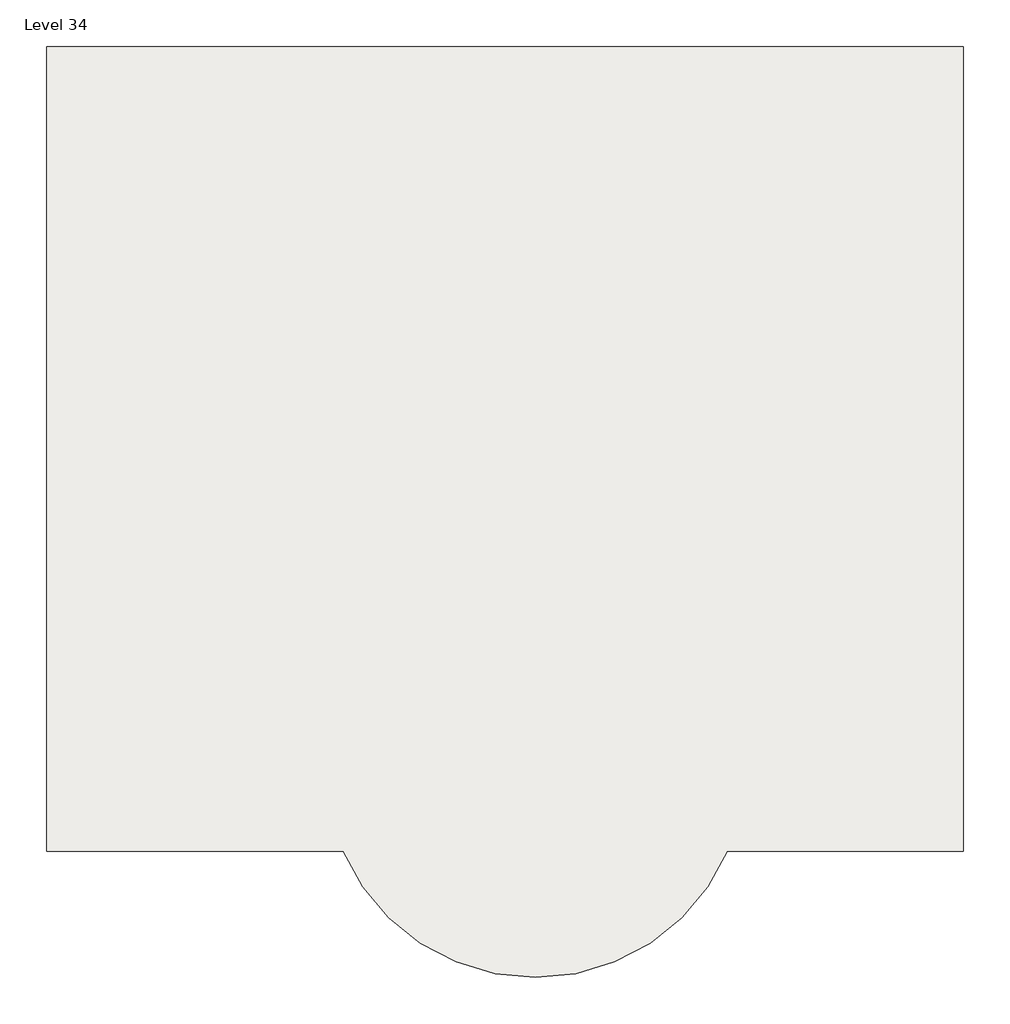
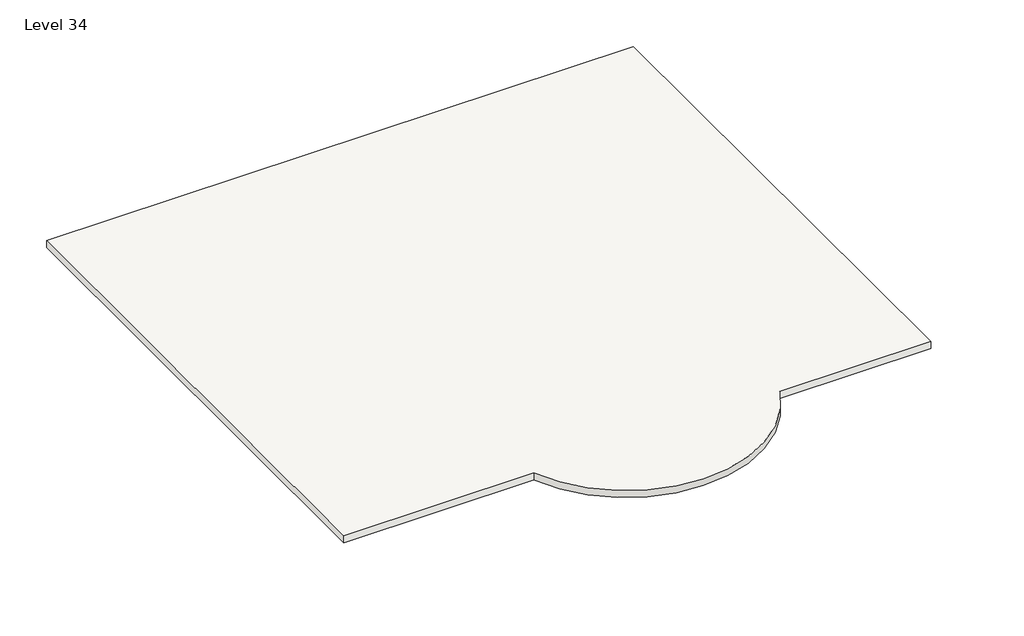
# One storey: 1 roof.
"""IFC4 building model written with IfcOpenShell, lengths in millimetres."""

from ifc_helpers import new_model, si_unit, point, frame, frame_2d, origin, place, context, project, spatial, polyline, circle_curve, trimmed, segment, composite_curve, outline, extrude, element, save

model = new_model("IFC4")

# Units and contexts
model_context = context("Model", 3, world=origin())
ifc_project = project(units=[si_unit("LENGTHUNIT", "METRE", prefix="MILLI")], contexts=[model_context])

# Site, building, storey
site = spatial("IfcSite", under=ifc_project)
building = spatial("IfcBuilding", under=site)
storey = spatial("IfcBuildingStorey", under=building, Name="Level 34", Elevation=55473.6)

# Roof
placement = place(None, origin())
element("IfcRoof", 1, ObjectType="Generic - 12\"", at=placement, inside=storey, context=model_context, shape_type="SweptSolid", body=[
    extrude(outline(composite_curve([segment(polyline([(-16556.2150607, 7359.5191779), (7928.4494573, 7359.5191779), (7928.4494573, -14128.8808221), (1626.8565143, -14128.8808221)]), True, "CONTINUOUS"), segment(trimmed(circle_curve(frame_2d((-3502.2792732, -11912.8408523)), 5587.3846363), [point((1626.8565143, -14128.8808221))], [point((-8631.4150607, -14128.8808221))], False, "CARTESIAN"), True, "CONTINUOUS"), segment(polyline([(-8631.4150607, -14128.8808221), (-16556.2150607, -14128.8808221), (-16556.2150607, 7359.5191779)]), True, "CONTINUOUS")], self_intersect=False)), frame((0.0, 0.0, 55473.6), z_axis=(0.0, 0.0, 1.0), x_axis=(1.0, 0.0, 0.0)), (0.0, 0.0, 1.0), 304.8),
])

save(model, "model.ifc")

# Revit data of these elements
# Type "Generic - 12\""
#   Assembly Code = "B1020"
#   Layers, outside or top first: 1' - 0" no material (function 1)
# Element 1 (IfcRoof, "Generic - 12\"")
#   built-in parameter 1001705 = 183 (stored number, unit not read)
#   built-in parameter 1001710 = 33615
#   Phase Created = New Construction
#   Materials on its faces: "Default Roof"
# Materials
#   "Default Roof": colour RGB 88 101 114, transparency 0
